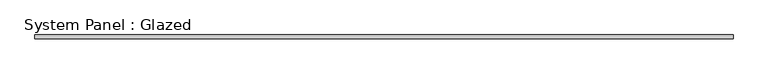
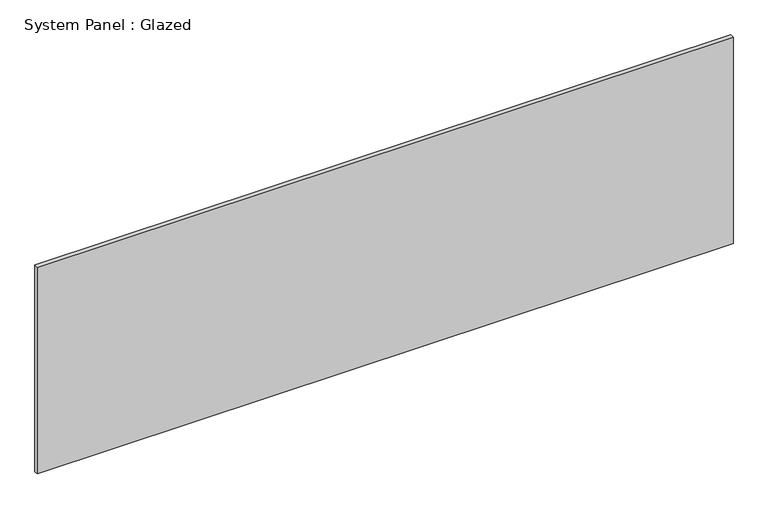
"""IFC4 building model written with IfcOpenShell, lengths in millimetres: plate geometry, System Panel : Glazed."""

from ifc_helpers import new_model, si_unit, origin, origin_with_axes, place, context, project, spatial, polyline, outline, extrude, source, transform, mapped, element, save


def system_panel_glazed_1f759628(model_context):
    return source(origin(), model_context, "Body", "SweptSolid", [
        extrude(outline(polyline([(2324.1, 19.05), (-2324.1, 19.05), (-2324.1, 44.45), (2324.1, 44.45), (2324.1, 19.05)])), origin_with_axes(), (0.0, 0.0, 1.0), 1460.5),
    ])


if __name__ == "__main__":
    model = new_model("IFC4")
    model_context = context("Model", 3, world=origin())
    ifc_project = project(units=[si_unit("LENGTHUNIT", "METRE", prefix="MILLI")], contexts=[model_context])
    site = spatial("IfcSite", under=ifc_project)
    building = spatial("IfcBuilding", under=site)
    placement = place(None, origin())
    system_panel_glazed_shape = system_panel_glazed_1f759628(model_context)
    element("IfcPlate", 1, ObjectType="System Panel : Glazed", at=placement, inside=building, context=model_context, shape_type="MappedRepresentation", body=[
        mapped(system_panel_glazed_shape, transform((0.0, 0.0, 0.0), x_axis=(1.0, 0.0, 0.0), y_axis=(0.0, 1.0, 0.0), z_axis=(0.0, 0.0, 1.0))),
    ])
    save(model, "model.ifc")

# Revit data of these elements
# Type "System Panel : Glazed"
#   Construction Type Id = "GSP4R"
#   Analytic Construction = "1/8 in Pilkington single glazing"
#   Visual Light Transmittance = 0.9
#   Solar Heat Gain Coefficient = 0.86
#   Heat Transfer Coefficient (U) = 1.18115 BTU/(h·ft²·°F)
# Element 1 (IfcPlate, "System Panel : Glazed")
#   Materials on its faces: "Glass"
# Materials
#   "Glass": class "Glass", colour RGB 0 128 192, transparency 0.75, Description = "Soda Lime Glass", Cost = 0
